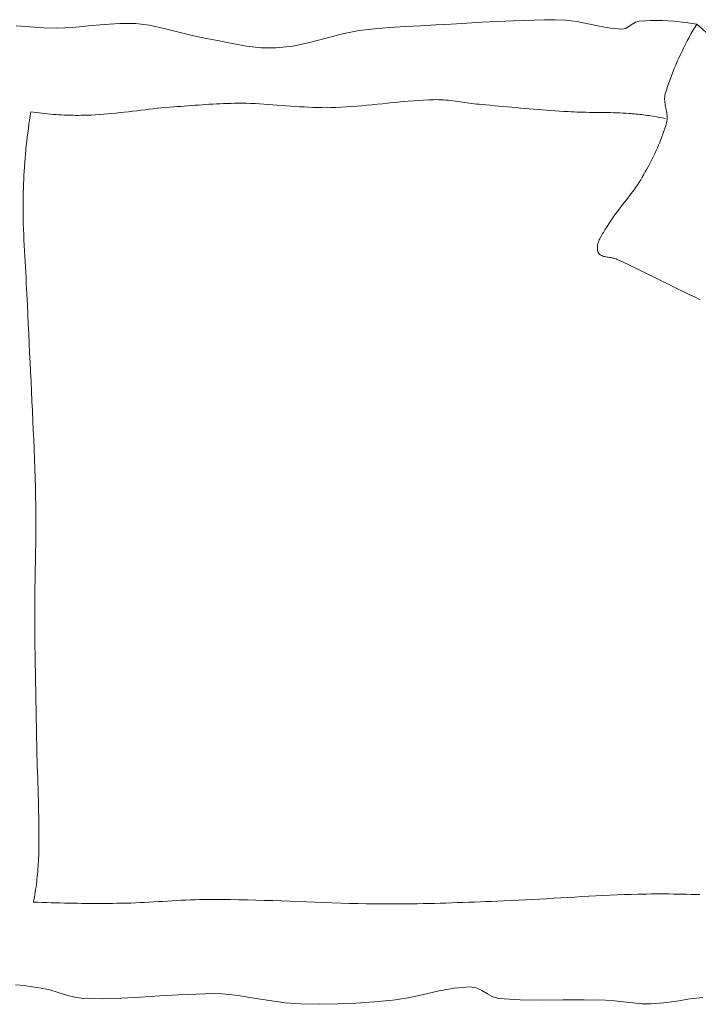
# Model space of a CAD drawing. Units: inches. Extents: x -36302355 to 648, y -221479757 to 75.
# Tile 17 of 37: x 516 to 555, y -530 to -473. Entities that reach past the tile are written whole.
import ezdxf

# ---------------------------------------------------------------- set-up
doc = ezdxf.new("R2010")
doc.units = ezdxf.units.IN
doc.header["$MEASUREMENT"] = 0
doc.layers.add('A-FURN', color=8, linetype='Continuous', lineweight=13)

# ---------------------------------------------------------------- blocks, each defined once
blk = doc.blocks.new('BED-DOUBLE')
for p, q in [((1, 46.159), (0.249, 45.317)), ((15.832, 45.216), (15.975, 45.513)), ((49.893, 45.241), (49.899, 45.492)), ((55.854, 44.918), (55.763, 45.66)), ((0.249, 45.317), (0.154, 44.664)), ((0.249, 45.317), (0.437, 45.204)), ((0.437, 45.204), (0.625, 45.093)), ((0.625, 45.093), (0.815, 44.985)), ((0.815, 44.985), (1.007, 44.879)), ((15.689, 44.919), (15.832, 45.216)), ((49.881, 44.738), (49.887, 44.989)), ((49.887, 44.989), (49.893, 45.241)), ((0.154, 44.664), (0.089, 44.006)), ((1.007, 44.879), (1.2, 44.776)), ((1.2, 44.776), (1.394, 44.675)), ((1.394, 44.675), (1.59, 44.576)), ((1.59, 44.576), (1.787, 44.479)), ((1.787, 44.479), (1.985, 44.386)), ((1.985, 44.386), (2.185, 44.294)), ((15.4, 44.327), (15.545, 44.623)), ((15.545, 44.623), (15.689, 44.919)), ((49.872, 44.235), (49.876, 44.487)), ((49.876, 44.487), (49.881, 44.738)), ((55.971, 44.178), (55.854, 44.918)), ((0.089, 44.006), (0.055, 43.345)), ((2.185, 44.294), (2.385, 44.205)), ((2.385, 44.205), (2.587, 44.119)), ((2.587, 44.119), (2.789, 44.035)), ((2.789, 44.035), (2.993, 43.954)), ((2.993, 43.954), (3.198, 43.875)), ((3.198, 43.875), (3.403, 43.799)), ((15.109, 43.736), (15.255, 44.031)), ((15.255, 44.031), (15.4, 44.327)), ((49.866, 43.733), (49.868, 43.984)), ((49.868, 43.984), (49.872, 44.235)), ((56.076, 43.436), (55.971, 44.178)), ((0.055, 43.345), (0.053, 42.684)), ((3.403, 43.799), (3.609, 43.726)), ((3.609, 43.726), (3.816, 43.655)), ((3.816, 43.655), (4.024, 43.587)), ((4.024, 43.587), (4.233, 43.522)), ((4.233, 43.522), (4.312, 43.502)), ((4.312, 43.502), (4.392, 43.489)), ((4.392, 43.489), (4.473, 43.482)), ((4.473, 43.482), (4.554, 43.482)), ((4.554, 43.482), (4.636, 43.486)), ((4.636, 43.486), (4.719, 43.494)), ((4.719, 43.494), (4.802, 43.505)), ((4.802, 43.505), (4.885, 43.519)), ((4.885, 43.519), (4.969, 43.535)), ((4.969, 43.535), (5.052, 43.552)), ((5.052, 43.552), (5.136, 43.569)), ((5.136, 43.569), (5.22, 43.585)), ((5.22, 43.585), (5.303, 43.599)), ((5.303, 43.599), (5.386, 43.611)), ((5.386, 43.611), (5.469, 43.621)), ((5.469, 43.621), (5.552, 43.626)), ((5.552, 43.626), (5.634, 43.627)), ((5.594, 43.326), (5.575, 43.223)), ((5.615, 43.43), (5.594, 43.326)), ((5.636, 43.533), (5.615, 43.43)), ((5.634, 43.627), (5.715, 43.622)), ((5.715, 43.622), (5.795, 43.611)), ((5.795, 43.611), (5.875, 43.593)), ((5.875, 43.593), (6.038, 43.546)), ((6.038, 43.546), (6.201, 43.496)), ((6.201, 43.496), (6.362, 43.443)), ((6.362, 43.443), (6.523, 43.387)), ((6.523, 43.387), (6.683, 43.329)), ((6.683, 43.329), (6.841, 43.268)), ((6.841, 43.268), (6.999, 43.204)), ((14.817, 43.145), (14.963, 43.44)), ((14.963, 43.44), (15.109, 43.736)), ((49.863, 43.23), (49.864, 43.481)), ((49.864, 43.481), (49.866, 43.733)), ((56.134, 42.692), (56.076, 43.436)), ((0.053, 42.684), (0.081, 42.025)), ((5.486, 42.703), (5.47, 42.599)), ((5.502, 42.808), (5.486, 42.703)), ((5.519, 42.912), (5.502, 42.808)), ((5.537, 43.015), (5.519, 42.912)), ((5.555, 43.119), (5.537, 43.015)), ((5.575, 43.223), (5.555, 43.119)), ((6.999, 43.204), (7.157, 43.138)), ((7.157, 43.138), (7.313, 43.07)), ((7.313, 43.07), (7.468, 43)), ((7.468, 43), (7.623, 42.928)), ((7.623, 42.928), (7.777, 42.854)), ((7.777, 42.854), (7.93, 42.778)), ((7.93, 42.778), (8.082, 42.701)), ((8.082, 42.701), (8.234, 42.622)), ((14.526, 42.554), (14.672, 42.849)), ((14.672, 42.849), (14.817, 43.145)), ((49.863, 42.979), (49.863, 43.23)), ((49.865, 42.727), (49.863, 42.979)), ((49.868, 42.476), (49.865, 42.727)), ((56.124, 42.175), (56.134, 42.692)), ((5.415, 42.181), (5.403, 42.077)), ((5.428, 42.286), (5.415, 42.181)), ((5.441, 42.39), (5.428, 42.286)), ((5.455, 42.495), (5.441, 42.39)), ((5.47, 42.599), (5.455, 42.495)), ((8.234, 42.622), (8.384, 42.542)), ((8.384, 42.542), (8.534, 42.46)), ((8.534, 42.46), (8.683, 42.378)), ((8.683, 42.378), (8.832, 42.295)), ((8.832, 42.295), (8.98, 42.21)), ((8.98, 42.21), (9.128, 42.123)), ((9.128, 42.123), (9.274, 42.031)), ((14.237, 41.962), (14.381, 42.258)), ((14.381, 42.258), (14.526, 42.554)), ((49.872, 42.225), (49.868, 42.476)), ((49.878, 41.973), (49.872, 42.225)), ((56.078, 41.659), (56.124, 42.175)), ((0.081, 42.025), (0.139, 41.819)), ((0.139, 41.819), (0.255, 41.628)), ((0.255, 41.628), (0.387, 41.441)), ((5.362, 41.657), (5.353, 41.552)), ((5.371, 41.762), (5.362, 41.657)), ((5.381, 41.867), (5.371, 41.762)), ((5.392, 41.972), (5.381, 41.867)), ((5.403, 42.077), (5.392, 41.972)), ((9.274, 42.031), (9.418, 41.936)), ((9.418, 41.936), (9.561, 41.838)), ((9.561, 41.838), (9.701, 41.738)), ((9.701, 41.738), (9.84, 41.635)), ((9.84, 41.635), (9.978, 41.531)), ((13.95, 41.369), (14.093, 41.666)), ((14.093, 41.666), (14.237, 41.962)), ((49.889, 41.571), (49.878, 41.973)), ((49.903, 41.169), (49.889, 41.571)), ((56.015, 41.144), (56.078, 41.659)), ((0.387, 41.441), (0.496, 41.249)), ((0.54, 41.043), (0.489, 40.398)), ((0.496, 41.249), (0.54, 41.043)), ((5.325, 41.1), (5.317, 40.926)), ((5.334, 41.274), (5.325, 41.1)), ((5.346, 41.447), (5.334, 41.274)), ((5.353, 41.552), (5.346, 41.447)), ((9.978, 41.531), (10.115, 41.425)), ((10.115, 41.425), (10.252, 41.319)), ((10.252, 41.319), (10.388, 41.212)), ((10.388, 41.212), (10.524, 41.105)), ((10.524, 41.105), (10.661, 40.998)), ((10.661, 40.998), (10.798, 40.892)), ((13.668, 40.774), (13.808, 41.071)), ((13.808, 41.071), (13.95, 41.369)), ((49.918, 40.767), (49.903, 41.169)), ((55.955, 40.628), (56.015, 41.144)), ((5.305, 40.579), (5.301, 40.405)), ((5.311, 40.753), (5.305, 40.579)), ((5.317, 40.926), (5.311, 40.753)), ((10.798, 40.892), (10.935, 40.786)), ((10.935, 40.786), (11.074, 40.683)), ((11.074, 40.683), (11.213, 40.581)), ((11.213, 40.581), (11.354, 40.481)), ((11.354, 40.481), (11.497, 40.385)), ((13.57, 40.401), (13.581, 40.468)), ((13.581, 40.468), (13.594, 40.534)), ((13.594, 40.534), (13.608, 40.598)), ((13.608, 40.598), (13.625, 40.659)), ((13.625, 40.659), (13.645, 40.718)), ((13.645, 40.718), (13.668, 40.774)), ((49.935, 40.364), (49.918, 40.767)), ((55.918, 40.112), (55.955, 40.628)), ((0.489, 40.398), (0.377, 39.758)), ((5.293, 39.883), (5.291, 39.709)), ((5.295, 40.057), (5.293, 39.883)), ((5.298, 40.231), (5.295, 40.057)), ((5.301, 40.405), (5.298, 40.231)), ((11.497, 40.385), (11.642, 40.291)), ((11.642, 40.291), (11.789, 40.201)), ((11.789, 40.201), (11.856, 40.16)), ((11.856, 40.16), (11.923, 40.118)), ((11.923, 40.118), (11.991, 40.075)), ((11.991, 40.075), (12.061, 40.031)), ((12.061, 40.031), (12.131, 39.988)), ((12.131, 39.988), (12.201, 39.944)), ((12.201, 39.944), (12.273, 39.902)), ((12.273, 39.902), (12.345, 39.86)), ((13.433, 39.847), (13.458, 39.897)), ((13.458, 39.897), (13.48, 39.952)), ((13.48, 39.952), (13.498, 40.01)), ((13.498, 40.01), (13.513, 40.071)), ((13.513, 40.071), (13.527, 40.135)), ((13.527, 40.135), (13.539, 40.2)), ((13.539, 40.2), (13.549, 40.267)), ((13.549, 40.267), (13.56, 40.334)), ((13.56, 40.334), (13.57, 40.401)), ((49.954, 39.962), (49.935, 40.364)), ((49.974, 39.56), (49.954, 39.962)), ((55.898, 38.895), (55.918, 40.112)), ((0.377, 39.758), (0.24, 39.119)), ((5.287, 39.361), (5.284, 39.187)), ((5.289, 39.535), (5.287, 39.361)), ((5.291, 39.709), (5.289, 39.535)), ((12.345, 39.86), (12.418, 39.821)), ((12.418, 39.821), (12.491, 39.785)), ((12.491, 39.785), (12.564, 39.752)), ((12.564, 39.752), (12.638, 39.722)), ((12.638, 39.722), (12.712, 39.696)), ((12.712, 39.696), (12.786, 39.675)), ((12.786, 39.675), (12.86, 39.659)), ((12.86, 39.659), (12.934, 39.649)), ((12.934, 39.649), (13.008, 39.646)), ((13.008, 39.646), (13.082, 39.649)), ((13.082, 39.649), (13.156, 39.659)), ((13.156, 39.659), (13.229, 39.677)), ((13.229, 39.677), (13.282, 39.698)), ((13.282, 39.698), (13.328, 39.726)), ((13.328, 39.726), (13.369, 39.761)), ((13.369, 39.761), (13.403, 39.801)), ((13.403, 39.801), (13.433, 39.847)), ((49.996, 39.159), (49.974, 39.56)), ((0.24, 39.119), (0.112, 38.48)), ((5.278, 38.839), (5.274, 38.666)), ((5.282, 39.013), (5.278, 38.839)), ((5.284, 39.187), (5.282, 39.013)), ((50.018, 38.757), (49.996, 39.159)), ((50.04, 38.355), (50.018, 38.757)), ((55.907, 37.677), (55.898, 38.895)), ((0.112, 38.48), (0.028, 37.836)), ((5.262, 38.318), (5.254, 38.144)), ((5.268, 38.492), (5.262, 38.318)), ((5.274, 38.666), (5.268, 38.492)), ((50.064, 37.953), (50.04, 38.355)), ((0.028, 37.836), (0, 37.235)), ((5.229, 37.723), (5.213, 37.476)), ((5.244, 37.971), (5.229, 37.723)), ((5.254, 38.144), (5.244, 37.971)), ((50.087, 37.551), (50.064, 37.953)), ((55.917, 36.459), (55.907, 37.677)), ((0, 37.235), (0, 36.634)), ((5.196, 37.228), (5.178, 36.981)), ((5.213, 37.476), (5.196, 37.228)), ((50.111, 37.149), (50.087, 37.551)), ((50.134, 36.747), (50.111, 37.149)), ((0, 36.634), (0.018, 36.032)), ((5.159, 36.734), (5.14, 36.487)), ((5.178, 36.981), (5.159, 36.734)), ((50.157, 36.345), (50.134, 36.747)), ((0.018, 36.032), (0.045, 35.43)), ((5.1, 35.992), (5.08, 35.745)), ((5.12, 36.239), (5.1, 35.992)), ((5.14, 36.487), (5.12, 36.239)), ((50.179, 35.943), (50.157, 36.345)), ((50.201, 35.542), (50.179, 35.943)), ((55.897, 35.242), (55.917, 36.459)), ((0.045, 35.43), (0.071, 34.828)), ((5.058, 35.498), (5.037, 35.251)), ((5.08, 35.745), (5.058, 35.498)), ((50.222, 35.14), (50.201, 35.542)), ((0.071, 34.828), (0.107, 33.948)), ((5.015, 35.004), (4.993, 34.757)), ((5.037, 35.251), (5.015, 35.004)), ((50.241, 34.737), (50.222, 35.14)), ((55.818, 34.029), (55.897, 35.242)), ((4.949, 34.263), (4.926, 34.016)), ((4.971, 34.51), (4.949, 34.263)), ((4.993, 34.757), (4.971, 34.51)), ((50.259, 34.335), (50.241, 34.737)), ((50.275, 33.933), (50.259, 34.335)), ((0.107, 33.948), (0.149, 33.068)), ((4.904, 33.769), (4.882, 33.522)), ((4.926, 34.016), (4.904, 33.769)), ((50.287, 33.608), (50.275, 33.933)), ((55.726, 33.689), (55.818, 34.029)), ((4.859, 33.275), (4.837, 33.028)), ((4.882, 33.522), (4.859, 33.275)), ((50.3, 33.282), (50.287, 33.608)), ((50.312, 32.957), (50.3, 33.282)), ((55.37, 33.05), (55.558, 33.367)), ((55.558, 33.367), (55.726, 33.689)), ((0.149, 33.068), (0.196, 32.188)), ((4.793, 32.623), (4.776, 32.487)), ((4.809, 32.758), (4.793, 32.623)), ((4.824, 32.893), (4.809, 32.758)), ((4.837, 33.028), (4.824, 32.893)), ((50.325, 32.632), (50.312, 32.957)), ((50.337, 32.306), (50.325, 32.632)), ((55.16, 32.385), (55.219, 32.726)), ((55.219, 32.726), (55.37, 33.05)), ((0.196, 32.188), (0.247, 31.308)), ((4.719, 32.082), (4.7, 31.947)), ((4.739, 32.217), (4.719, 32.082)), ((4.758, 32.352), (4.739, 32.217)), ((4.776, 32.487), (4.758, 32.352)), ((50.348, 31.981), (50.337, 32.306)), ((55.234, 31.495), (55.16, 32.385)), ((4.644, 31.542), (4.627, 31.407)), ((4.662, 31.677), (4.644, 31.542)), ((4.681, 31.812), (4.662, 31.677)), ((4.7, 31.947), (4.681, 31.812)), ((50.36, 31.655), (50.348, 31.981)), ((50.371, 31.33), (50.36, 31.655)), ((55.394, 30.613), (55.234, 31.495)), ((0.247, 31.308), (0.302, 30.429)), ((4.586, 31.001), (4.576, 30.866)), ((4.598, 31.136), (4.586, 31.001)), ((4.612, 31.272), (4.598, 31.136)), ((4.627, 31.407), (4.612, 31.272)), ((50.381, 31.004), (50.371, 31.33)), ((50.39, 30.679), (50.381, 31.004)), ((0.302, 30.429), (0.351, 29.554)), ((4.563, 30.595), (4.561, 30.459)), ((4.561, 30.459), (4.562, 30.323)), ((4.568, 30.73), (4.563, 30.595)), ((4.576, 30.866), (4.568, 30.73)), ((50.399, 30.353), (50.39, 30.679)), ((50.408, 30.028), (50.399, 30.353)), ((55.593, 29.734), (55.394, 30.613)), ((4.562, 30.323), (4.57, 30.028)), ((4.57, 30.028), (4.583, 29.734)), ((50.415, 29.702), (50.408, 30.028)), ((0.351, 29.554), (0.396, 28.679)), ((4.583, 29.734), (4.601, 29.439)), ((4.601, 29.439), (4.621, 29.145)), ((50.421, 29.376), (50.415, 29.702)), ((50.426, 29.051), (50.421, 29.376)), ((55.784, 28.854), (55.593, 29.734)), ((0.396, 28.679), (0.448, 27.804)), ((4.621, 29.145), (4.645, 28.851)), ((4.645, 28.851), (4.671, 28.557)), ((50.43, 28.725), (50.426, 29.051)), ((50.433, 28.4), (50.43, 28.725)), ((55.919, 27.967), (55.784, 28.854)), ((4.671, 28.557), (4.699, 28.263)), ((4.699, 28.263), (4.728, 27.969)), ((50.435, 28.074), (50.433, 28.4)), ((0.448, 27.804), (0.521, 26.932)), ((4.728, 27.969), (4.759, 27.675)), ((4.759, 27.675), (4.79, 27.382)), ((50.434, 27.423), (50.435, 27.749)), ((50.435, 27.749), (50.435, 28.074)), ((56.015, 26.923), (55.919, 27.967)), ((4.79, 27.382), (4.821, 27.088)), ((4.821, 27.088), (4.852, 26.794)), ((50.429, 26.939), (50.434, 27.423)), ((0.521, 26.932), (0.625, 26.063)), ((4.852, 26.794), (4.881, 26.5)), ((4.881, 26.5), (4.909, 26.207)), ((50.412, 25.97), (50.422, 26.454)), ((50.422, 26.454), (50.429, 26.939)), ((56.091, 25.876), (56.015, 26.923)), ((0.625, 26.063), (0.809, 25.109)), ((4.909, 26.207), (4.935, 25.913)), ((4.935, 25.913), (4.958, 25.618)), ((50.399, 25.486), (50.412, 25.97)), ((56.14, 24.828), (56.091, 25.876)), ((4.958, 25.618), (4.978, 25.324)), ((4.978, 25.324), (4.995, 25.03)), ((50.385, 25.001), (50.399, 25.486)), ((0.809, 25.109), (1.05, 24.163)), ((4.995, 25.03), (5.007, 24.735)), ((5.007, 24.735), (5.015, 24.44)), ((50.37, 24.517), (50.385, 25.001)), ((56.158, 23.779), (56.14, 24.828)), ((1.05, 24.163), (1.298, 23.22)), ((5.015, 24.44), (5.018, 24.185)), ((5.018, 24.185), (5.016, 23.931)), ((50.353, 24.033), (50.37, 24.517)), ((5.011, 23.676), (5.002, 23.421)), ((5.016, 23.931), (5.011, 23.676)), ((50.336, 23.549), (50.353, 24.033)), ((56.139, 22.73), (56.158, 23.779)), ((1.298, 23.22), (1.501, 22.271)), ((4.991, 23.166), (4.977, 22.912)), ((5.002, 23.421), (4.991, 23.166)), ((50.299, 22.581), (50.317, 23.065)), ((50.317, 23.065), (50.336, 23.549)), ((4.961, 22.657), (4.943, 22.403)), ((4.977, 22.912), (4.961, 22.657)), ((50.281, 22.096), (50.299, 22.581)), ((56.069, 21.831), (56.139, 22.73)), ((1.501, 22.271), (1.61, 21.31)), ((4.924, 22.148), (4.905, 21.894)), ((4.943, 22.403), (4.924, 22.148)), ((50.263, 21.612), (50.281, 22.096)), ((4.866, 21.385), (4.847, 21.13)), ((4.885, 21.639), (4.866, 21.385)), ((4.905, 21.894), (4.885, 21.639)), ((50.245, 21.128), (50.263, 21.612)), ((55.946, 20.936), (56.069, 21.831)), ((1.61, 21.31), (1.596, 20.47)), ((4.829, 20.876), (4.812, 20.621)), ((4.847, 21.13), (4.829, 20.876)), ((50.229, 20.644), (50.245, 21.128)), ((55.8, 20.042), (55.946, 20.936)), ((1.596, 20.47), (1.501, 19.634)), ((4.798, 20.366), (4.785, 20.111)), ((4.812, 20.621), (4.798, 20.366)), ((50.215, 20.16), (50.229, 20.644)), ((4.776, 19.857), (4.77, 19.602)), ((4.785, 20.111), (4.776, 19.857)), ((50.19, 19.191), (50.201, 19.676)), ((50.201, 19.676), (50.215, 20.16)), ((55.663, 19.148), (55.8, 20.042)), ((1.501, 19.634), (1.355, 18.801)), ((4.77, 19.602), (4.767, 19.347)), ((4.767, 19.347), (4.767, 19.142)), ((4.767, 19.142), (4.77, 18.938)), ((50.182, 18.707), (50.19, 19.191)), ((55.566, 18.25), (55.663, 19.148)), ((1.355, 18.801), (1.187, 17.969)), ((4.77, 18.938), (4.773, 18.733)), ((4.773, 18.733), (4.779, 18.528)), ((50.176, 18.223), (50.182, 18.707)), ((4.779, 18.528), (4.786, 18.323)), ((4.786, 18.323), (4.794, 18.119)), ((4.794, 18.119), (4.803, 17.914)), ((50.173, 17.738), (50.176, 18.223)), ((55.546, 17.754), (55.566, 18.25)), ((1.187, 17.969), (1.029, 17.139)), ((4.803, 17.914), (4.814, 17.71)), ((4.814, 17.71), (4.826, 17.505)), ((4.826, 17.505), (4.838, 17.301)), ((50.174, 17.476), (50.173, 17.738)), ((50.177, 17.214), (50.174, 17.476)), ((55.553, 17.258), (55.546, 17.754)), ((1.029, 17.139), (0.867, 16.371)), ((4.838, 17.301), (4.852, 17.096)), ((4.852, 17.096), (4.866, 16.892)), ((4.866, 16.892), (4.88, 16.688)), ((50.183, 16.952), (50.177, 17.214)), ((50.192, 16.69), (50.183, 16.952)), ((55.576, 16.762), (55.553, 17.258)), ((0.867, 16.371), (0.673, 15.608)), ((4.88, 16.688), (4.895, 16.483)), ((4.895, 16.483), (4.911, 16.279)), ((50.202, 16.429), (50.192, 16.69)), ((50.214, 16.167), (50.202, 16.429)), ((55.604, 16.266), (55.576, 16.762)), ((4.911, 16.279), (4.927, 16.075)), ((4.927, 16.075), (4.943, 15.87)), ((4.943, 15.87), (4.959, 15.666)), ((50.227, 15.905), (50.214, 16.167)), ((50.241, 15.643), (50.227, 15.905)), ((55.626, 15.769), (55.604, 16.266)), ((55.678, 14.678), (55.626, 15.769)), ((0.673, 15.608), (0.479, 14.846)), ((4.959, 15.666), (4.975, 15.462)), ((4.975, 15.462), (4.991, 15.258)), ((4.991, 15.258), (5.01, 15.021)), ((50.256, 15.381), (50.241, 15.643)), ((50.272, 15.12), (50.256, 15.381)), ((0.479, 14.846), (0.317, 14.08)), ((5.01, 15.021), (5.032, 14.784)), ((5.032, 14.784), (5.055, 14.547)), ((50.287, 14.858), (50.272, 15.12)), ((50.303, 14.596), (50.287, 14.858)), ((55.747, 13.587), (55.678, 14.678)), ((0.317, 14.08), (0.222, 13.304)), ((5.055, 14.547), (5.08, 14.31)), ((5.08, 14.31), (5.106, 14.074)), ((5.106, 14.074), (5.133, 13.837)), ((50.319, 14.334), (50.303, 14.596)), ((50.333, 14.073), (50.319, 14.334)), ((50.347, 13.811), (50.333, 14.073)), ((5.133, 13.837), (5.161, 13.601)), ((5.161, 13.601), (5.189, 13.364)), ((50.36, 13.549), (50.347, 13.811)), ((50.371, 13.287), (50.36, 13.549)), ((55.809, 12.496), (55.747, 13.587)), ((0.222, 13.304), (0.211, 12.406)), ((5.189, 13.364), (5.218, 13.128)), ((5.218, 13.128), (5.246, 12.892)), ((50.381, 13.025), (50.371, 13.287)), ((50.388, 12.763), (50.381, 13.025)), ((0.211, 12.406), (0.269, 11.508)), ((5.246, 12.892), (5.273, 12.655)), ((5.273, 12.655), (5.3, 12.419)), ((5.3, 12.419), (5.325, 12.182)), ((50.394, 12.501), (50.388, 12.763)), ((50.397, 12.25), (50.394, 12.501)), ((55.842, 11.405), (55.809, 12.496)), ((5.325, 12.182), (5.349, 11.946)), ((5.349, 11.946), (5.372, 11.709)), ((50.4, 11.999), (50.397, 12.25)), ((50.402, 11.747), (50.4, 11.999)), ((0.269, 11.508), (0.358, 10.61)), ((5.372, 11.709), (5.392, 11.472)), ((5.392, 11.472), (5.41, 11.235)), ((5.41, 11.235), (5.425, 10.998)), ((50.403, 11.496), (50.402, 11.747)), ((50.404, 11.244), (50.403, 11.496)), ((50.404, 10.993), (50.404, 11.244)), ((55.821, 10.315), (55.842, 11.405)), ((5.425, 10.998), (5.438, 10.76)), ((5.438, 10.76), (5.447, 10.523)), ((50.402, 10.49), (50.403, 10.742)), ((50.403, 10.742), (50.404, 10.993)), ((0.358, 10.61), (0.444, 9.712)), ((5.447, 10.523), (5.452, 10.363)), ((5.452, 10.363), (5.454, 10.202)), ((5.454, 10.202), (5.456, 10.042)), ((50.397, 9.987), (50.4, 10.239)), ((50.4, 10.239), (50.402, 10.49)), ((55.755, 9.827), (55.821, 10.315)), ((0.444, 9.712), (0.487, 8.812)), ((5.451, 9.56), (5.446, 9.399)), ((5.454, 9.721), (5.451, 9.56)), ((5.456, 9.881), (5.454, 9.721)), ((5.456, 10.042), (5.456, 9.881)), ((50.389, 9.485), (50.393, 9.736)), ((50.393, 9.736), (50.397, 9.987)), ((55.631, 9.348), (55.755, 9.827)), ((5.432, 9.078), (5.422, 8.918)), ((5.44, 9.239), (5.432, 9.078)), ((5.446, 9.399), (5.44, 9.239)), ((50.379, 8.982), (50.384, 9.233)), ((50.384, 9.233), (50.389, 9.485)), ((55.479, 8.873), (55.631, 9.348)), ((0.487, 8.812), (0.469, 8.039)), ((5.385, 8.437), (5.37, 8.278)), ((5.399, 8.598), (5.385, 8.437)), ((5.412, 8.758), (5.399, 8.598)), ((5.422, 8.918), (5.412, 8.758)), ((50.357, 8.228), (50.365, 8.479)), ((50.365, 8.479), (50.372, 8.731)), ((50.372, 8.731), (50.379, 8.982)), ((55.334, 8.396), (55.479, 8.873)), ((0.469, 8.039), (0.415, 7.265)), ((5.335, 7.958), (5.315, 7.799)), ((5.353, 8.118), (5.335, 7.958)), ((5.37, 8.278), (5.353, 8.118)), ((50.34, 7.726), (50.349, 7.977)), ((50.349, 7.977), (50.357, 8.228)), ((55.153, 7.423), (55.228, 7.912)), ((55.228, 7.912), (55.334, 8.396)), ((5.27, 7.481), (5.246, 7.323)), ((5.246, 7.323), (5.486, 7.284)), ((5.293, 7.64), (5.27, 7.481)), ((5.315, 7.799), (5.293, 7.64)), ((19.558, 7.278), (20.107, 7.305)), ((20.107, 7.305), (20.656, 7.332)), ((20.656, 7.332), (21.206, 7.359)), ((21.206, 7.359), (21.755, 7.385)), ((21.755, 7.385), (22.304, 7.411)), ((22.304, 7.411), (22.853, 7.436)), ((22.853, 7.436), (23.402, 7.461)), ((23.402, 7.461), (23.952, 7.484)), ((23.952, 7.484), (24.501, 7.507)), ((24.501, 7.507), (25.05, 7.528)), ((25.05, 7.528), (25.6, 7.547)), ((25.6, 7.547), (26.149, 7.565)), ((26.149, 7.565), (26.698, 7.581)), ((26.698, 7.581), (27.248, 7.595)), ((27.248, 7.595), (27.588, 7.602)), ((27.588, 7.602), (27.927, 7.606)), ((27.927, 7.606), (28.267, 7.609)), ((28.267, 7.609), (28.607, 7.609)), ((28.607, 7.609), (28.946, 7.608)), ((28.946, 7.608), (29.286, 7.605)), ((29.286, 7.605), (29.626, 7.602)), ((29.626, 7.602), (29.966, 7.597)), ((29.966, 7.597), (30.305, 7.592)), ((30.305, 7.592), (30.645, 7.586)), ((30.645, 7.586), (30.985, 7.579)), ((30.985, 7.579), (31.325, 7.573)), ((31.325, 7.573), (31.664, 7.566)), ((31.664, 7.566), (32.004, 7.56)), ((32.004, 7.56), (32.344, 7.555)), ((32.344, 7.555), (32.684, 7.55)), ((32.684, 7.55), (33.023, 7.546)), ((33.023, 7.546), (33.363, 7.544)), ((33.363, 7.544), (33.703, 7.543)), ((33.703, 7.543), (34.043, 7.543)), ((34.043, 7.543), (34.39, 7.545)), ((34.39, 7.545), (34.737, 7.547)), ((34.737, 7.547), (35.085, 7.55)), ((35.085, 7.55), (35.432, 7.554)), ((35.432, 7.554), (35.779, 7.558)), ((35.779, 7.558), (36.127, 7.563)), ((36.127, 7.563), (36.474, 7.568)), ((36.474, 7.568), (36.821, 7.573)), ((36.821, 7.573), (37.168, 7.579)), ((37.168, 7.579), (37.516, 7.585)), ((37.516, 7.585), (37.863, 7.591)), ((37.863, 7.591), (38.21, 7.598)), ((38.21, 7.598), (38.558, 7.604)), ((38.558, 7.604), (38.905, 7.611)), ((38.905, 7.611), (39.252, 7.618)), ((39.252, 7.618), (39.599, 7.625)), ((39.599, 7.625), (39.947, 7.631)), ((39.947, 7.631), (40.294, 7.638)), ((40.294, 7.638), (40.641, 7.644)), ((40.641, 7.644), (40.989, 7.65)), ((40.989, 7.65), (41.309, 7.657)), ((41.309, 7.657), (41.63, 7.664)), ((41.63, 7.664), (41.951, 7.672)), ((41.951, 7.672), (42.272, 7.681)), ((42.272, 7.681), (42.593, 7.691)), ((42.593, 7.691), (42.914, 7.701)), ((42.914, 7.701), (43.235, 7.712)), ((43.235, 7.712), (43.556, 7.722)), ((43.556, 7.722), (43.877, 7.732)), ((43.877, 7.732), (44.198, 7.742)), ((44.198, 7.742), (44.519, 7.751)), ((44.519, 7.751), (44.839, 7.76)), ((44.839, 7.76), (45.16, 7.767)), ((45.16, 7.767), (45.481, 7.773)), ((45.481, 7.773), (45.802, 7.778)), ((45.802, 7.778), (46.123, 7.782)), ((46.123, 7.782), (46.444, 7.783)), ((46.444, 7.783), (46.765, 7.783)), ((46.765, 7.783), (47.086, 7.78)), ((47.086, 7.78), (47.407, 7.776)), ((47.407, 7.776), (47.554, 7.772)), ((47.554, 7.772), (47.701, 7.768)), ((47.701, 7.768), (47.847, 7.762)), ((47.847, 7.762), (47.994, 7.755)), ((47.994, 7.755), (48.141, 7.746)), ((48.141, 7.746), (48.288, 7.737)), ((48.288, 7.737), (48.435, 7.726)), ((48.435, 7.726), (48.582, 7.714)), ((48.582, 7.714), (48.728, 7.701)), ((48.728, 7.701), (48.875, 7.686)), ((48.875, 7.686), (49.021, 7.671)), ((49.021, 7.671), (49.167, 7.654)), ((49.167, 7.654), (49.313, 7.635)), ((49.313, 7.635), (49.459, 7.616)), ((49.459, 7.616), (49.605, 7.596)), ((49.605, 7.596), (49.75, 7.574)), ((49.75, 7.574), (49.896, 7.551)), ((49.896, 7.551), (50.041, 7.527)), ((50.041, 7.527), (50.185, 7.501)), ((50.185, 7.501), (50.33, 7.475)), ((50.33, 7.475), (50.34, 7.726)), ((55.086, 6.932), (55.153, 7.423)), ((0.415, 7.265), (0.354, 6.492)), ((5.486, 7.284), (5.727, 7.247)), ((5.727, 7.247), (5.968, 7.212)), ((5.968, 7.212), (6.21, 7.179)), ((6.21, 7.179), (6.451, 7.147)), ((6.451, 7.147), (6.693, 7.117)), ((6.693, 7.117), (6.935, 7.089)), ((6.935, 7.089), (7.178, 7.062)), ((7.178, 7.062), (7.42, 7.038)), ((7.42, 7.038), (7.663, 7.015)), ((7.663, 7.015), (7.906, 6.994)), ((7.906, 6.994), (8.149, 6.974)), ((8.149, 6.974), (8.392, 6.956)), ((8.392, 6.956), (8.635, 6.941)), ((8.635, 6.941), (8.879, 6.927)), ((8.879, 6.927), (9.122, 6.914)), ((9.122, 6.914), (9.365, 6.904)), ((9.365, 6.904), (9.609, 6.895)), ((9.609, 6.895), (9.852, 6.888)), ((9.852, 6.888), (10.096, 6.883)), ((10.096, 6.883), (10.404, 6.879)), ((10.404, 6.879), (10.713, 6.878)), ((10.713, 6.878), (11.021, 6.88)), ((11.021, 6.88), (11.33, 6.886)), ((11.33, 6.886), (11.638, 6.893)), ((11.638, 6.893), (11.947, 6.903)), ((11.947, 6.903), (12.255, 6.914)), ((12.255, 6.914), (12.563, 6.928)), ((12.563, 6.928), (12.872, 6.942)), ((12.872, 6.942), (13.18, 6.958)), ((13.18, 6.958), (13.488, 6.975)), ((13.488, 6.975), (13.796, 6.993)), ((13.796, 6.993), (14.105, 7.011)), ((14.105, 7.011), (14.413, 7.029)), ((14.413, 7.029), (14.721, 7.047)), ((14.721, 7.047), (15.03, 7.064)), ((15.03, 7.064), (15.338, 7.081)), ((15.338, 7.081), (15.646, 7.097)), ((15.646, 7.097), (15.955, 7.112)), ((15.955, 7.112), (16.263, 7.126)), ((16.263, 7.126), (16.812, 7.149)), ((16.812, 7.149), (17.361, 7.174)), ((17.361, 7.174), (17.911, 7.199)), ((17.911, 7.199), (18.46, 7.225)), ((18.46, 7.225), (19.009, 7.251)), ((19.009, 7.251), (19.558, 7.278)), ((55.042, 6.439), (55.086, 6.932))]:
    blk.add_line(p, q)

msp = doc.modelspace()

# ---------------------------------------------------------------- block references
at = {"layer": 'A-FURN', "rotation": 270}
msp.add_blockref('BED-DOUBLE', (509.53, -473.482), dxfattribs=at)

doc.saveas('drawing.dxf')
